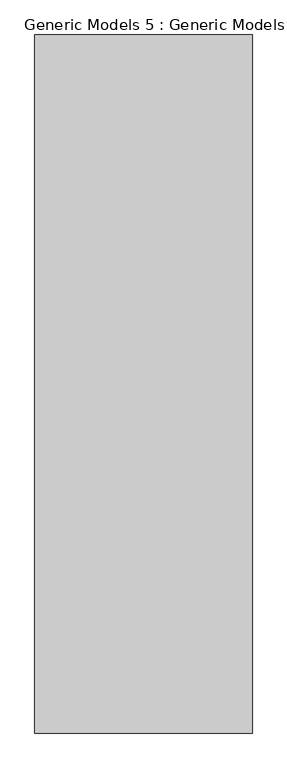
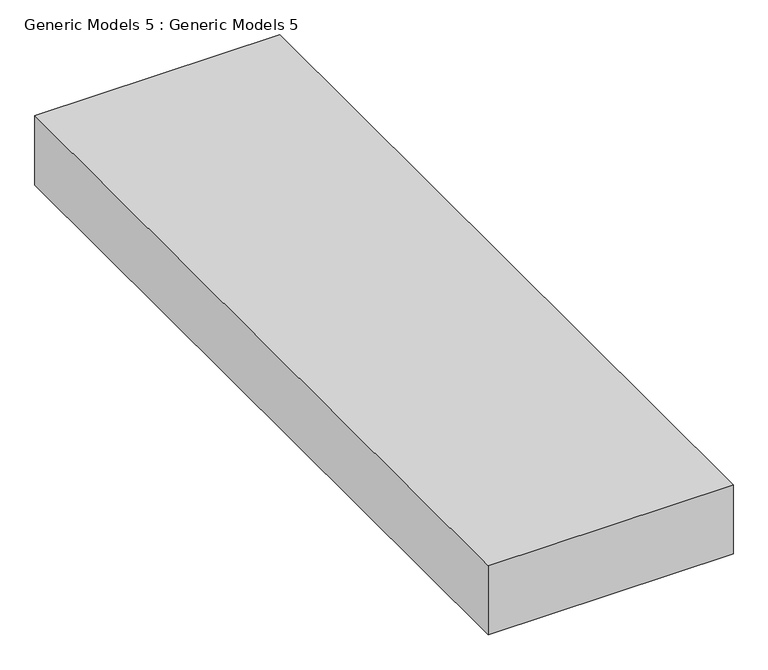
"""IFC4 building model written with IfcOpenShell, lengths in millimetres: proxy geometry, Generic Models 5 : Generic Models 5."""

from ifc_helpers import new_model, si_unit, frame, origin, place, context, project, spatial, polyline, outline, extrude, source, transform, mapped, element, save


def generic_models_5_generic_models_5_415a3505(model_context):
    return source(origin(), model_context, "Body", "SweptSolid", [
        extrude(outline(polyline([(-10330.5247823, -11256.0546119), (-10841.7386697, -11256.0546119), (-10841.7386697, -9616.2611111), (-10330.5247823, -9616.2611111), (-10330.5247823, -11256.0546119)])), frame((0.0, 0.0, 5551.780974), z_axis=(0.0, 0.0, 1.0), x_axis=(1.0, 0.0, 0.0)), (0.0, 0.0, 1.0), 152.4),
    ])


if __name__ == "__main__":
    model = new_model("IFC4")
    model_context = context("Model", 3, world=origin())
    ifc_project = project(units=[si_unit("LENGTHUNIT", "METRE", prefix="MILLI")], contexts=[model_context])
    site = spatial("IfcSite", under=ifc_project)
    building = spatial("IfcBuilding", under=site)
    placement = place(None, origin())
    generic_models_5_generic_models_5_shape = generic_models_5_generic_models_5_415a3505(model_context)
    element("IfcBuildingElementProxy", 1, Name="Generic Models 5 : Generic Models 5", ObjectType="Generic Models 5 : Generic Models 5", at=placement, inside=building, context=model_context, shape_type="MappedRepresentation", body=[
        mapped(generic_models_5_generic_models_5_shape, transform((0.0, 0.0, 0.0), x_axis=(1.0, 0.0, 0.0), y_axis=(0.0, 1.0, 0.0), z_axis=(0.0, 0.0, 1.0))),
    ])
    save(model, "model.ifc")
